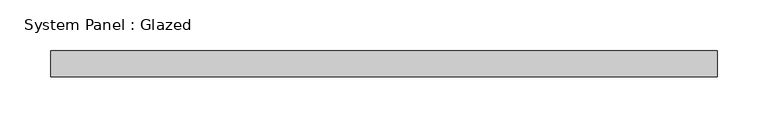
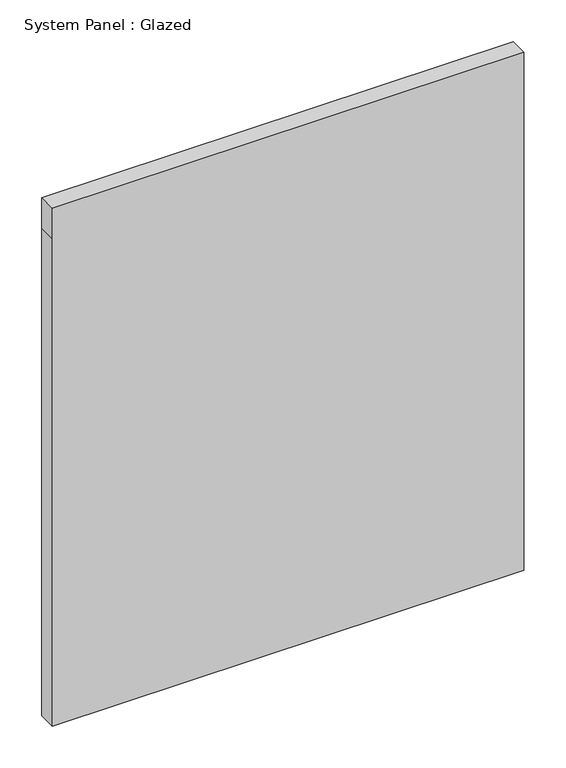
"""IFC4 building model written with IfcOpenShell, lengths in millimetres: plate geometry, System Panel : Glazed."""

from ifc_helpers import new_model, si_unit, frame, origin, place, context, project, spatial, polyline, outline, extrude, source, transform, mapped, element, save


def system_panel_glazed_2cf72723(model_context):
    return source(origin(), model_context, "Body", "SweptSolid", [
        extrude(outline(polyline([(0.0, -327.0977679), (0.0, 327.0977679), (714.926051, 327.0977679), (759.376051, 327.0977679), (759.376051, -327.0977679), (714.926051, -327.0977679), (0.0, -327.0977679)])), frame((0.0, 19.05, 0.0), z_axis=(0.0, 1.0, 0.0), x_axis=(0.0, 0.0, 1.0)), (0.0, 0.0, 1.0), 25.4),
    ])


if __name__ == "__main__":
    model = new_model("IFC4")
    model_context = context("Model", 3, world=origin())
    ifc_project = project(units=[si_unit("LENGTHUNIT", "METRE", prefix="MILLI")], contexts=[model_context])
    site = spatial("IfcSite", under=ifc_project)
    building = spatial("IfcBuilding", under=site)
    placement = place(None, origin())
    system_panel_glazed_shape = system_panel_glazed_2cf72723(model_context)
    element("IfcPlate", 1, ObjectType="System Panel : Glazed", at=placement, inside=building, context=model_context, shape_type="MappedRepresentation", body=[
        mapped(system_panel_glazed_shape, transform((0.0, 0.0, 0.0), x_axis=(1.0, 0.0, 0.0), y_axis=(0.0, 1.0, 0.0), z_axis=(0.0, 0.0, 1.0))),
    ])
    save(model, "model.ifc")

# Revit data of these elements
# Type "System Panel : Glazed"
#   Construction Type Id = "GSP4R"
#   Analytic Construction = "1/8 in Pilkington single glazing"
#   Visual Light Transmittance = 0.9
#   Solar Heat Gain Coefficient = 0.86
#   Heat Transfer Coefficient (U) = 1.18115 BTU/(h·ft²·°F)
#   Define Thermal Properties by = 1
# Element 1 (IfcPlate, "System Panel : Glazed")
#   Materials on its faces: "Glass"
# Materials
#   "Glass": class "Glass", colour RGB 0 128 192, transparency 0.75, Description = "Soda Lime Glass", Cost = 0
